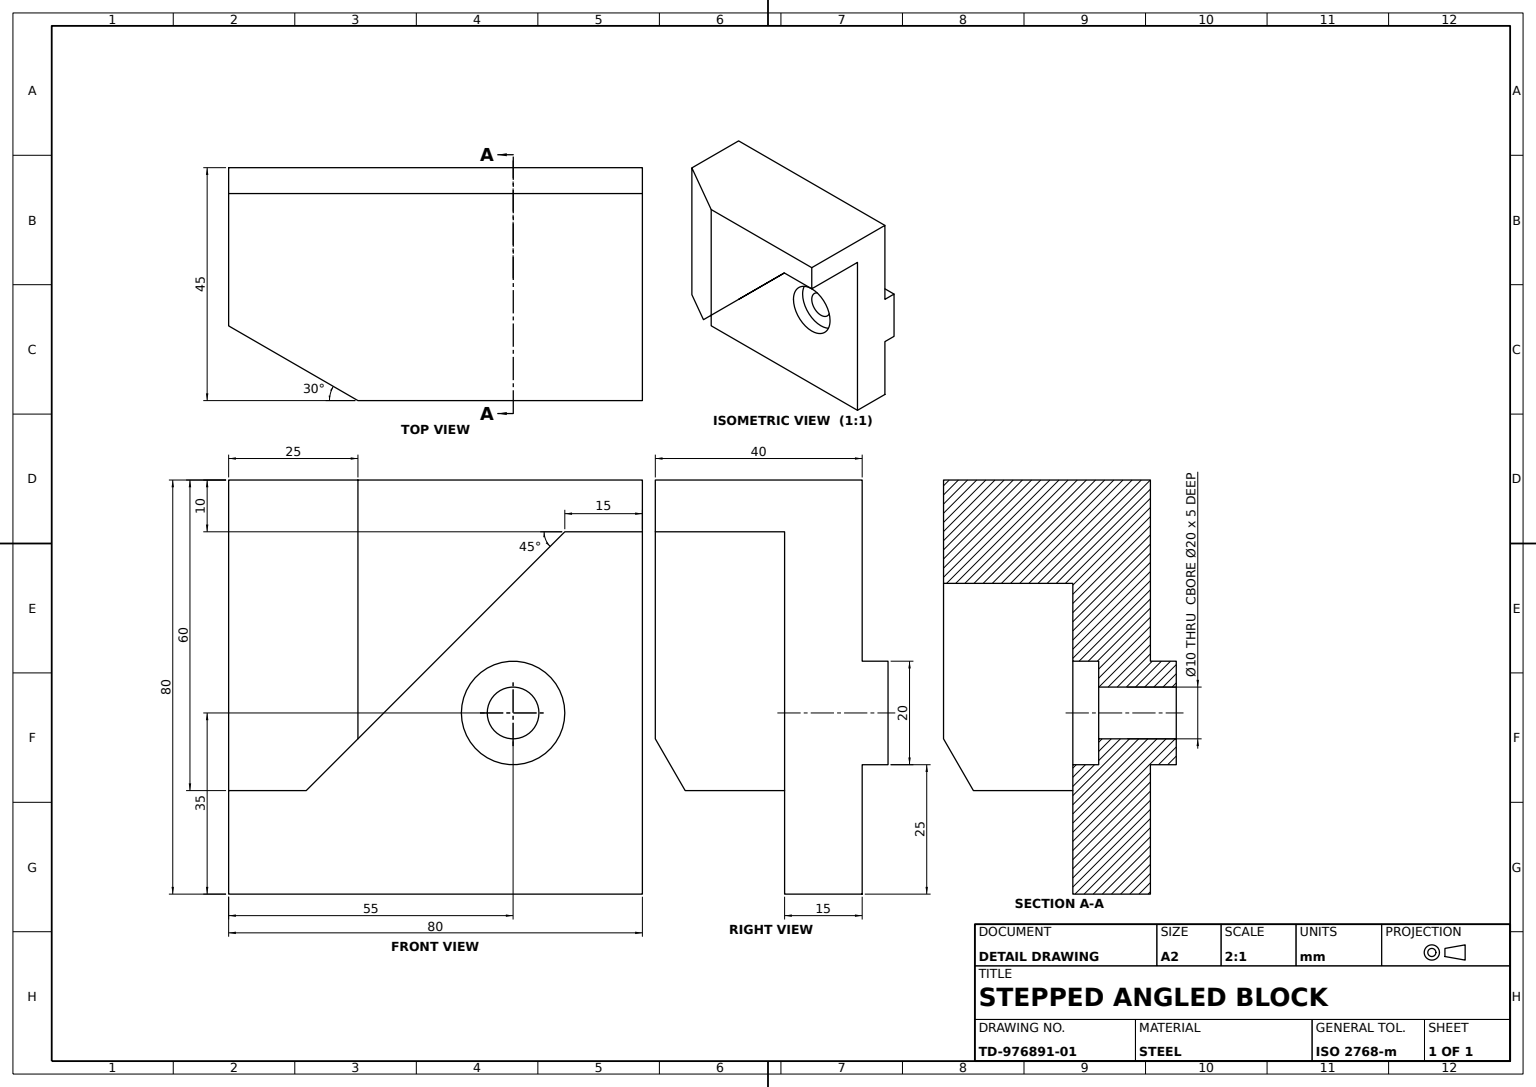
from build123d import *

# Parameters (mm, degrees)
BASE_PLATE_SKETCH_W       = 80
BASE_PLATE_SKETCH_H       = 80
BASE_PLATE_80X80X15_DEPTH = 15
VERTICAL_WALL_SKETCH_W    = 5
VERTICAL_WALL_SKETCH_H    = 20
VERTICAL_WALL_DEPTH       = 80
STEP_BOSS_SKETCH_W        = 55
STEP_BOSS_SKETCH_H        = 25
STEP_BOSS_DEPTH           = 10
V_BLOCK_BODY_DEPTH        = 60
ANGLED_BOSS_45DEG_DEPTH   = 25
V_GROOVE_CUT_DEPTH        = 25
COUNTERBORE_SKETCH_R      = 10
COUNTERBORE_20X5_DEPTH    = 5
HOLE_SKETCH_R             = 5
HOLE_10_DEPTH             = 20


with BuildPart() as part:
    # Base Plate Sketch → Base Plate 80x80x15 (new body)
    with BuildSketch(Plane.XY):
        with Locations((40, -40)):
            Rectangle(BASE_PLATE_SKETCH_W, BASE_PLATE_SKETCH_H)
    extrude(amount=BASE_PLATE_80X80X15_DEPTH)

    # Vertical Wall Sketch → Vertical Wall (add)
    with BuildSketch(Plane(origin=(80, 0, 0), x_dir=(0, 0, -1), z_dir=(1, 0, 0))):
        with Locations((2.5, -45)):
            Rectangle(VERTICAL_WALL_SKETCH_W, VERTICAL_WALL_SKETCH_H)
    extrude(amount=-VERTICAL_WALL_DEPTH)

    # Step Boss Sketch → Step Boss (add)
    with BuildSketch(Plane(origin=(0, 0, 0), x_dir=(1, 0, 0), z_dir=(0, 1, 0))):
        with Locations((52.5, -27.5)):
            Rectangle(STEP_BOSS_SKETCH_W, STEP_BOSS_SKETCH_H)
    extrude(amount=-STEP_BOSS_DEPTH)

    # V Block Body Sketch → V Block Body (add)
    with BuildSketch(Plane(origin=(0, 0, 0), x_dir=(1, 0, 0), z_dir=(0, 1, 0))):
        Polygon((25, -40), (0, -25.56624327), (0, -15), (25, -15), align=None)
    extrude(amount=-V_BLOCK_BODY_DEPTH)

    # Angled Boss 45deg Sketch → Angled Boss 45deg (add)
    with BuildSketch(Plane.XY.offset(40)):
        Polygon((65, -10), (31.374324096, -43.625675904), (25, -50), (25, -10), align=None)
    extrude(amount=-ANGLED_BOSS_45DEG_DEPTH)

    # V Groove Sketch → V Groove Cut (cut)
    with BuildSketch(Plane.XY.offset(40)):
        Polygon((25, -50), (15, -60), (25, -60), align=None)
    extrude(amount=-V_GROOVE_CUT_DEPTH, mode=Mode.SUBTRACT)

    # Counterbore Sketch → Counterbore Ø20x5 (cut)
    with BuildSketch(Plane.XY.offset(15)):
        with Locations((55, -45)):
            Circle(COUNTERBORE_SKETCH_R)
    extrude(amount=-COUNTERBORE_20X5_DEPTH, mode=Mode.SUBTRACT)

    # Hole Sketch → Hole Ø10 (cut)
    with BuildSketch(Plane.XY.offset(10)):
        with Locations((55, -45)):
            Circle(HOLE_SKETCH_R)
    extrude(amount=-HOLE_10_DEPTH, mode=Mode.SUBTRACT)


solid = part.part
